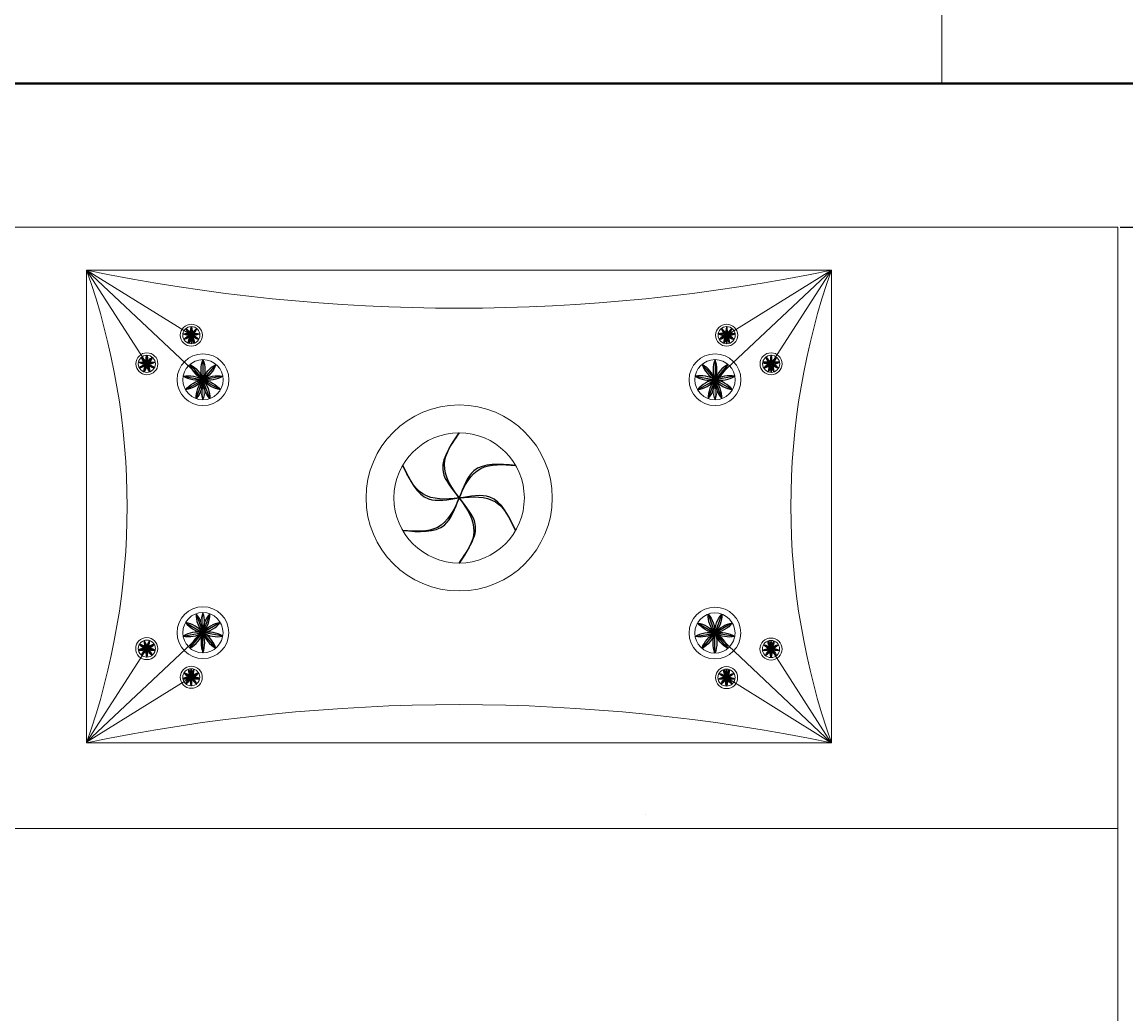
# Model space of a CAD drawing. Units: inches. Extents: x -46 to 1145, y -527 to 760.
# Tile 41 of 57: x 83 to 114, y 625 to 652. Entities that reach past the tile are written whole.
import ezdxf

# ---------------------------------------------------------------- set-up
doc = ezdxf.new("R2010")
doc.units = ezdxf.units.IN
doc.header["$MEASUREMENT"] = 0
for name, color, linetype, lineweight in [('A-ANNO-DIMS', 2, 'Continuous', 18), ('A-FURN', 2, 'Continuous', 13), ('WALLS', 4, 'Continuous', 40), ('WINDOWS', 240, 'Continuous', 20)]:
    doc.layers.add(name, color=color, linetype=linetype, lineweight=lineweight)
doc.layers.add('FURNTIURE', color=2, linetype='Continuous')
doc.layers.add('LT', color=9, linetype='Continuous')
doc.styles.get("Standard").update_dxf_attribs({"font": 'arial.ttf'})
doc.dimstyles.get("Standard").update_dxf_attribs({"dimtxt": 0.18, "dimasz": 0.18, "dimexe": 0.18, "dimexo": 0.0625, "dimgap": 0.09, "dimtad": 0, "dimtih": 1, "dimtoh": 1, "dimdec": 0, "dimzin": 0, "dimdsep": 46, "dimlunit": 3, "dimtxsty": 'Standard', "dimcen": 0.09, "dimadec": 0, "dimazin": 0, "dimtfac": 1, "dimtdec": 0, "dimtofl": 0, "dimtmove": 0, "dimatfit": 3, "dimfxl": 1, "dimtolj": 1, "dimtzin": 0, "dimarcsym": 0})

# ---------------------------------------------------------------- blocks, each defined once
blk = doc.blocks.new('WINDOW-36IN')
blk.add_line((36, 9), (36, 0))
blk = doc.blocks.new('*U58')
at = {"layer": 'LT'}
blk.add_line((0, 0.281), (0, -0.281), dxfattribs=at)
for centre, start, end in [((0.734, 0), 159.0676, 200.9324), ((-0.734, 0), 339.0676, 20.9324)]:
    blk.add_arc(centre, 0.786, start, end, dxfattribs=at)
blk = doc.blocks.new('*U59')
at = {"layer": 'LT', "transparency": 16777216}
for p, rotation in [((609.756, 443.96), 40.00000000000002), ((610.117, 443.96), 320), ((609.659, 443.794), 80.00000000000001), ((610.213, 443.794), 280), ((609.693, 443.605), 120), ((609.84, 443.481), 160), ((610.032, 443.481), 200), ((610.179, 443.605), 240)]:
    blk.add_blockref('*U58', p, dxfattribs=dict(at, rotation=rotation))
blk.add_blockref('*U58', (609.936, 444.026), dxfattribs=at)
blk = doc.blocks.new('*U60')
at = {"layer": 'LT'}
blk.add_line((0, 0.12), (0, -0.12), dxfattribs=at)
for centre, start, end in [((0.313, 0), 159.0676, 200.9324), ((-0.313, 0), 339.0676, 20.9324)]:
    blk.add_arc(centre, 0.335, start, end, dxfattribs=at)
blk = doc.blocks.new('*U61')
at = {"layer": 'LT', "transparency": 16777216}
for p, rotation in [((259.536, 188.967), 40), ((259.69, 188.967), 320), ((259.495, 188.896), 80.00000000000001), ((259.509, 188.816), 120), ((259.572, 188.763), 160), ((259.654, 188.763), 200), ((259.716, 188.816), 240), ((259.731, 188.896), 280)]:
    blk.add_blockref('*U60', p, dxfattribs=dict(at, rotation=rotation))
blk.add_blockref('*U60', (259.613, 188.995), dxfattribs=at)
blk = doc.blocks.new('*U62')
at = {"layer": 'LT'}
blk.add_line((0, 0.12), (0, -0.12), dxfattribs=at)
for centre, start, end in [((0.313, 0), 159.0676, 200.9324), ((-0.313, 0), 339.0676, 20.9324)]:
    blk.add_arc(centre, 0.335, start, end, dxfattribs=at)
blk = doc.blocks.new('*U63')
at = {"layer": 'LT', "transparency": 16777216}
for p, rotation in [((259.536, 188.967), 40), ((259.69, 188.967), 320), ((259.495, 188.896), 80.00000000000001), ((259.509, 188.816), 120), ((259.572, 188.763), 160), ((259.654, 188.763), 200), ((259.716, 188.816), 240), ((259.731, 188.896), 280)]:
    blk.add_blockref('*U62', p, dxfattribs=dict(at, rotation=rotation))
blk.add_blockref('*U62', (259.613, 188.995), dxfattribs=at)
blk = doc.blocks.new('*U64')
at = {"layer": 'LT'}
blk.add_line((0, 0.281), (0, -0.281), dxfattribs=at)
for centre, start, end in [((0.734, 0), 159.0676, 200.9324), ((-0.734, 0), 339.0676, 20.9324)]:
    blk.add_arc(centre, 0.786, start, end, dxfattribs=at)
blk = doc.blocks.new('*U65')
at = {"layer": 'LT', "transparency": 16777216}
for p, rotation in [((609.756, 443.96), 40.00000000000002), ((610.117, 443.96), 320), ((609.659, 443.794), 80.00000000000001), ((610.213, 443.794), 280), ((609.693, 443.605), 120), ((609.84, 443.481), 160), ((610.032, 443.481), 200), ((610.179, 443.605), 240)]:
    blk.add_blockref('*U64', p, dxfattribs=dict(at, rotation=rotation))
blk.add_blockref('*U64', (609.936, 444.026), dxfattribs=at)
blk = doc.blocks.new('*U66')
at = {"layer": 'LT'}
blk.add_line((0, 0.12), (0, -0.12), dxfattribs=at)
for centre, start, end in [((0.313, 0), 159.0676, 200.9324), ((-0.313, 0), 339.0676, 20.9324)]:
    blk.add_arc(centre, 0.335, start, end, dxfattribs=at)
blk = doc.blocks.new('*U67')
at = {"layer": 'LT', "transparency": 16777216}
for p, rotation in [((259.536, 188.967), 40), ((259.69, 188.967), 320), ((259.495, 188.896), 80.00000000000001), ((259.509, 188.816), 120), ((259.572, 188.763), 160), ((259.654, 188.763), 200), ((259.716, 188.816), 240), ((259.731, 188.896), 280)]:
    blk.add_blockref('*U66', p, dxfattribs=dict(at, rotation=rotation))
blk.add_blockref('*U66', (259.613, 188.995), dxfattribs=at)
blk = doc.blocks.new('*U68')
at = {"layer": 'LT'}
blk.add_line((0, 0.12), (0, -0.12), dxfattribs=at)
for centre, start, end in [((0.313, 0), 159.0676, 200.9324), ((-0.313, 0), 339.0676, 20.9324)]:
    blk.add_arc(centre, 0.335, start, end, dxfattribs=at)
blk = doc.blocks.new('*U69')
at = {"layer": 'LT', "transparency": 16777216}
for p, rotation in [((259.536, 188.967), 40), ((259.69, 188.967), 320), ((259.495, 188.896), 80.00000000000001), ((259.509, 188.816), 120), ((259.572, 188.763), 160), ((259.654, 188.763), 200), ((259.716, 188.816), 240), ((259.731, 188.896), 280)]:
    blk.add_blockref('*U68', p, dxfattribs=dict(at, rotation=rotation))
blk.add_blockref('*U68', (259.613, 188.995), dxfattribs=at)
blk = doc.blocks.new('*U70')
at = {"layer": 'LT'}
blk.add_line((0, 0.281), (0, -0.281), dxfattribs=at)
for centre, start, end in [((0.734, 0), 159.0676, 200.9324), ((-0.734, 0), 339.0676, 20.9324)]:
    blk.add_arc(centre, 0.786, start, end, dxfattribs=at)
blk = doc.blocks.new('*U71')
at = {"layer": 'LT', "transparency": 16777216}
for p, rotation in [((609.756, 443.96), 40.00000000000002), ((610.117, 443.96), 320), ((609.659, 443.794), 80.00000000000001), ((610.213, 443.794), 280), ((609.693, 443.605), 120), ((609.84, 443.481), 160), ((610.032, 443.481), 200), ((610.179, 443.605), 240)]:
    blk.add_blockref('*U70', p, dxfattribs=dict(at, rotation=rotation))
blk.add_blockref('*U70', (609.936, 444.026), dxfattribs=at)
blk = doc.blocks.new('*U46')
at = {"layer": 'LT'}
blk.add_line((0, 0.12), (0, -0.12), dxfattribs=at)
for centre, start, end in [((0.313, 0), 159.0676, 200.9324), ((-0.313, 0), 339.0676, 20.9324)]:
    blk.add_arc(centre, 0.335, start, end, dxfattribs=at)
blk = doc.blocks.new('*U47')
at = {"layer": 'LT', "transparency": 16777216}
for p, rotation in [((259.536, 188.967), 40), ((259.69, 188.967), 320), ((259.495, 188.896), 80.00000000000001), ((259.509, 188.816), 120), ((259.572, 188.763), 160), ((259.654, 188.763), 200), ((259.716, 188.816), 240), ((259.731, 188.896), 280)]:
    blk.add_blockref('*U46', p, dxfattribs=dict(at, rotation=rotation))
blk.add_blockref('*U46', (259.613, 188.995), dxfattribs=at)
blk = doc.blocks.new('*U48')
at = {"layer": 'LT'}
blk.add_line((0, 0.12), (0, -0.12), dxfattribs=at)
for centre, start, end in [((0.313, 0), 159.0676, 200.9324), ((-0.313, 0), 339.0676, 20.9324)]:
    blk.add_arc(centre, 0.335, start, end, dxfattribs=at)
blk = doc.blocks.new('*U49')
at = {"layer": 'LT', "transparency": 16777216}
for p, rotation in [((259.536, 188.967), 40), ((259.69, 188.967), 320), ((259.495, 188.896), 80.00000000000001), ((259.509, 188.816), 120), ((259.572, 188.763), 160), ((259.654, 188.763), 200), ((259.716, 188.816), 240), ((259.731, 188.896), 280)]:
    blk.add_blockref('*U48', p, dxfattribs=dict(at, rotation=rotation))
blk.add_blockref('*U48', (259.613, 188.995), dxfattribs=at)
blk = doc.blocks.new('*U50')
at = {"layer": 'LT'}
blk.add_line((0, 0.281), (0, -0.281), dxfattribs=at)
for centre, start, end in [((0.734, 0), 159.0676, 200.9324), ((-0.734, 0), 339.0676, 20.9324)]:
    blk.add_arc(centre, 0.786, start, end, dxfattribs=at)
blk = doc.blocks.new('*U51')
at = {"layer": 'LT', "transparency": 16777216}
for p, rotation in [((609.756, 443.96), 40.00000000000002), ((610.117, 443.96), 320), ((609.659, 443.794), 80.00000000000001), ((610.213, 443.794), 280), ((609.693, 443.605), 120), ((609.84, 443.481), 160), ((610.032, 443.481), 200), ((610.179, 443.605), 240)]:
    blk.add_blockref('*U50', p, dxfattribs=dict(at, rotation=rotation))
blk.add_blockref('*U50', (609.936, 444.026), dxfattribs=at)
blk = doc.blocks.new('*U52')
at = {"layer": 'LT'}
blk.add_line((0, 0.12), (0, -0.12), dxfattribs=at)
for centre, start, end in [((0.313, 0), 159.0676, 200.9324), ((-0.313, 0), 339.0676, 20.9324)]:
    blk.add_arc(centre, 0.335, start, end, dxfattribs=at)
blk = doc.blocks.new('*U53')
at = {"layer": 'LT', "transparency": 16777216}
for p, rotation in [((259.536, 188.967), 40), ((259.69, 188.967), 320), ((259.495, 188.896), 80.00000000000001), ((259.509, 188.816), 120), ((259.572, 188.763), 160), ((259.654, 188.763), 200), ((259.716, 188.816), 240), ((259.731, 188.896), 280)]:
    blk.add_blockref('*U52', p, dxfattribs=dict(at, rotation=rotation))
blk.add_blockref('*U52', (259.613, 188.995), dxfattribs=at)
blk = doc.blocks.new('*U54')
at = {"layer": 'LT'}
blk.add_line((0, 0.12), (0, -0.12), dxfattribs=at)
for centre, start, end in [((0.313, 0), 159.0676, 200.9324), ((-0.313, 0), 339.0676, 20.9324)]:
    blk.add_arc(centre, 0.335, start, end, dxfattribs=at)
blk = doc.blocks.new('*U55')
at = {"layer": 'LT', "transparency": 16777216}
for p, rotation in [((259.536, 188.967), 40), ((259.69, 188.967), 320), ((259.495, 188.896), 80.00000000000001), ((259.509, 188.816), 120), ((259.572, 188.763), 160), ((259.654, 188.763), 200), ((259.716, 188.816), 240), ((259.731, 188.896), 280)]:
    blk.add_blockref('*U54', p, dxfattribs=dict(at, rotation=rotation))
blk.add_blockref('*U54', (259.613, 188.995), dxfattribs=at)
blk = doc.blocks.new('*U56')
at = {"layer": 'FURNTIURE'}
blk.add_open_spline([(0.039, 1.82), (-0.218, 1.447), (-0.661, 0.801), (0.102, -0.025), (0.645, -0.928), (0.238, -1.527), (0.039, -1.82)], degree=3, knots=[0, 0, 0, 0, 1.177175, 2.037162, 3.056205, 4.032246, 4.032246, 4.032246, 4.032246], dxfattribs=at)
blk = doc.blocks.new('*U57')
at = {"layer": 'FURNTIURE', "transparency": 16777216}
blk.add_blockref('*U56', (904.302, 663.383), dxfattribs=at)
for p, rotation in [((904.379, 663.383), 180), ((904.321, 663.416), 300), ((904.321, 663.349), 59.99999999999999), ((904.36, 663.416), 239.9999999999999), ((904.36, 663.349), 119.9999999999999)]:
    blk.add_blockref('*U56', p, dxfattribs=dict(at, rotation=rotation))
blk = doc.blocks.new('BED-QUEEN-FURNISHED')
for p, q in [((0, 80), (60, 80)), ((60, 80), (60, 0)), ((31.2, 78.8), (52, 78.8)), ((31.2, 65.6), (31.2, 78.8)), ((31.2, 78.8), (52, 78.8)), ((31.2, 65.6), (31.2, 78.8)), ((31.2, 78.8), (34.585, 75.613)), ((31.2, 78.8), (32.884, 76.184)), ((31.2, 78.8), (34.126, 76.984)), ((52, 78.8), (48.615, 75.613)), ((52, 78.8), (49.074, 76.984)), ((52, 78.8), (50.315, 76.184)), ((52, 78.8), (52, 65.6)), ((52, 78.8), (52, 65.6)), ((34.126, 76.984), (34.126, 76.745)), ((49.074, 76.984), (49.074, 76.745)), ((50.315, 76.184), (50.315, 75.945)), ((34.451, 75.739), (34.451, 75.177)), ((48.748, 75.739), (48.748, 75.177)), ((34.449, 68.673), (34.449, 69.235)), ((31.195, 65.614), (34.582, 68.799)), ((51.995, 65.6), (48.612, 68.789)), ((50.312, 68.216), (50.313, 68.456)), ((31.195, 65.614), (32.882, 68.228)), ((51.995, 65.6), (50.312, 68.216)), ((34.123, 67.428), (34.123, 67.667)), ((49.07, 67.418), (49.07, 67.657)), ((31.195, 65.614), (34.123, 67.428)), ((51.995, 65.6), (49.07, 67.418)), ((31.2, 65.6), (52, 65.6)), ((31.2, 65.6), (52, 65.6)), ((46.8, 63.6), (46.799, 63.6)), ((60, 63.2), (0, 63.2))]:
    blk.add_line(p, q)
for centre, radius in [((34.126, 76.984), 0.308), ((34.126, 76.984), 0.239), ((49.074, 76.984), 0.308), ((49.074, 76.984), 0.239), ((32.884, 76.184), 0.308), ((34.451, 75.739), 0.723), ((48.748, 75.739), 0.723), ((50.315, 76.184), 0.308), ((32.884, 76.184), 0.239), ((34.451, 75.739), 0.562), ((48.748, 75.739), 0.562), ((50.315, 76.184), 0.239), ((41.604, 72.437), 2.599), ((41.604, 72.437), 1.82), ((34.449, 68.673), 0.723), ((48.746, 68.663), 0.723), ((34.449, 68.673), 0.562), ((48.746, 68.663), 0.562), ((32.882, 68.228), 0.308), ((32.882, 68.228), 0.239), ((50.312, 68.216), 0.308), ((50.312, 68.216), 0.239), ((34.123, 67.428), 0.308), ((34.123, 67.428), 0.239), ((49.07, 67.418), 0.308), ((49.07, 67.418), 0.239)]:
    blk.add_circle(centre, radius)
for centre, radius, start, end in [((41.6, 129.177), 51.439, 258.3356, 281.6644), ((12.546, 72.2), 19.787, 340.5151, 19.4849), ((70.653, 72.2), 19.787, 160.5151, 199.4849), ((34.439, 76.865), 0.335, 159.0676, 200.9324), ((33.814, 76.865), 0.335, 339.0676, 20.9324), ((49.386, 76.865), 0.335, 159.0676, 200.9324), ((48.761, 76.865), 0.335, 339.0676, 20.9324), ((50.628, 76.065), 0.335, 159.0676, 200.9324), ((50.003, 76.065), 0.335, 339.0676, 20.9324), ((35.185, 75.458), 0.786, 159.0676, 200.9324), ((33.717, 75.458), 0.786, 339.0676, 20.9324), ((49.483, 75.458), 0.786, 159.0676, 200.9324), ((48.014, 75.458), 0.786, 339.0676, 20.9324), ((35.183, 68.953), 0.786, 159.028, 200.8928), ((33.715, 68.954), 0.786, 339.028, 20.8928), ((50.625, 68.336), 0.335, 159.028, 200.8928), ((50, 68.336), 0.335, 339.028, 20.8928), ((34.435, 67.547), 0.335, 159.028, 200.8928), ((33.81, 67.548), 0.335, 339.028, 20.8928), ((49.383, 67.537), 0.335, 159.028, 200.8928), ((48.758, 67.537), 0.335, 339.028, 20.8928), ((41.6, 15.223), 51.439, 78.3356, 101.6644)]:
    blk.add_arc(centre, radius, start, end)
at = {"xscale": -1}
for name, p in [('*U69', (293.739, -111.891)), ('*U67', (292.497, -112.691)), ('*U65', (644.387, -368.006))]:
    blk.add_blockref(name, p, dxfattribs=at)
for name, p in [('*U63', (-210.539, -111.891)), ('*U59', (-561.188, -368.006)), ('*U61', (-209.298, -112.691)), ('*U57', (-862.736, -590.946))]:
    blk.add_blockref(name, p)
at = {"rotation": 179.9603994254766}
for name, p in [('*U51', (644.691, 511.997)), ('*U53', (292.625, 256.925)), ('*U55', (293.866, 256.124))]:
    blk.add_blockref(name, p, dxfattribs=at)
at = {"xscale": -1, "rotation": 179.9603994254766}
for name, p in [('*U71', (-560.883, 512.83)), ('*U47', (-209.17, 257.271)), ('*U49', (-210.412, 256.472))]:
    blk.add_blockref(name, p, dxfattribs=at)
blk = doc.blocks.new('*D652')
at = {"layer": 'A-ANNO-DIMS', "color": 0, "lineweight": -2, "transparency": 16777216}
for p, q in [((113.972, 646.503), (126.09, 646.503)), ((125.91, 646.323), (125.91, 606.691)), ((125.91, 566.683), (125.91, 606.314)), ((113.972, 566.503), (126.09, 566.503))]:
    blk.add_line(p, q, dxfattribs=at)
at = {"layer": 'A-ANNO-DIMS', "color": 0, "transparency": 16777216}
for points in [[(125.88, 646.323), (125.94, 646.323), (125.91, 646.503)], [(125.88, 566.683), (125.94, 566.683), (125.91, 566.503)]]:
    blk.add_solid(points, dxfattribs=at)
at = {"layer": 'Defpoints', "color": 0, "transparency": 16777216}
for p in [(113.91, 646.503), (125.91, 646.503), (113.91, 566.503)]:
    blk.add_point(p, dxfattribs=at)
at = {"layer": 'A-ANNO-DIMS', "color": 0, "transparency": 16777216, "insert": (125.91, 606.503), "char_height": 0.18, "attachment_point": 5}
blk.add_mtext('\\A1;QUEEN BED 80 TYP.', dxfattribs=at)
blk = doc.blocks.new('*D685')
at = {"layer": 'A-ANNO-DIMS', "color": 0, "lineweight": -2, "transparency": 16777216}
for p, q in [((183.501, 700.889), (-46.216, 700.889)), ((-46.036, 700.709), (-46.036, 116.385)), ((-46.036, -468.302), (-46.036, 116.021)), ((12.501, -468.482), (-46.216, -468.482))]:
    blk.add_line(p, q, dxfattribs=at)
at = {"layer": 'A-ANNO-DIMS', "color": 0, "transparency": 16777216}
for points in [[(-46.066, 700.709), (-46.006, 700.709), (-46.036, 700.889)], [(-46.066, -468.302), (-46.006, -468.302), (-46.036, -468.482)]]:
    blk.add_solid(points, dxfattribs=at)
at = {"layer": 'Defpoints', "color": 0, "transparency": 16777216}
for p in [(-46.036, 700.889), (183.564, 700.889), (12.564, -468.482)]:
    blk.add_point(p, dxfattribs=at)
at = {"layer": 'A-ANNO-DIMS', "color": 0, "transparency": 16777216, "insert": (-46.036, 116.203), "char_height": 0.18, "attachment_point": 5}
blk.add_mtext('\\A1;1169.4', dxfattribs=at)

msp = doc.modelspace()

# ---------------------------------------------------------------- linework, layer by layer
at = {"layer": 'WALLS'}
msp.add_line((183.5637, 650.5176), (21.5637, 650.5176), dxfattribs=at)

# ---------------------------------------------------------------- block references
at = {"layer": 'A-FURN'}
msp.add_blockref('BED-QUEEN-FURNISHED', (53.91, 566.503), dxfattribs=at)
at = {"layer": 'WINDOWS'}
msp.add_blockref('WINDOW-36IN', (72.995, 650.518), dxfattribs=at)

# ---------------------------------------------------------------- dimensions: what is measured, and where the dimension line sits
at = {"layer": 'A-ANNO-DIMS'}
dim = msp.add_linear_dim(base=(-46.0363, 700.8886), p1=(12.5637, -468.4824), p2=(183.5637, 700.8886), angle=90, dimstyle='Standard', override={"dimdec": 1, "dimlfac": 1, "dimrnd": 0, "dimzin": 0, "dimdsep": 46, "dimlunit": 2}, dxfattribs=at)
dim.commit()
dim.dimension.update_dxf_attribs({"geometry": '*D685', "text_midpoint": (-46.0363, 116.2031)})
dim = msp.add_linear_dim(base=(125.9098, 646.5029), p1=(113.9098, 566.5028), p2=(113.9098, 646.5029), angle=90, text='QUEEN BED <> TYP.', dimstyle='Standard', override={"dimdec": 0, "dimlfac": 1, "dimrnd": 0, "dimzin": 0, "dimdsep": 46, "dimlunit": 2}, dxfattribs=at)
dim.commit()
dim.dimension.update_dxf_attribs({"geometry": '*D652', "text_midpoint": (125.9098, 606.5028)})

doc.saveas('drawing.dxf')
